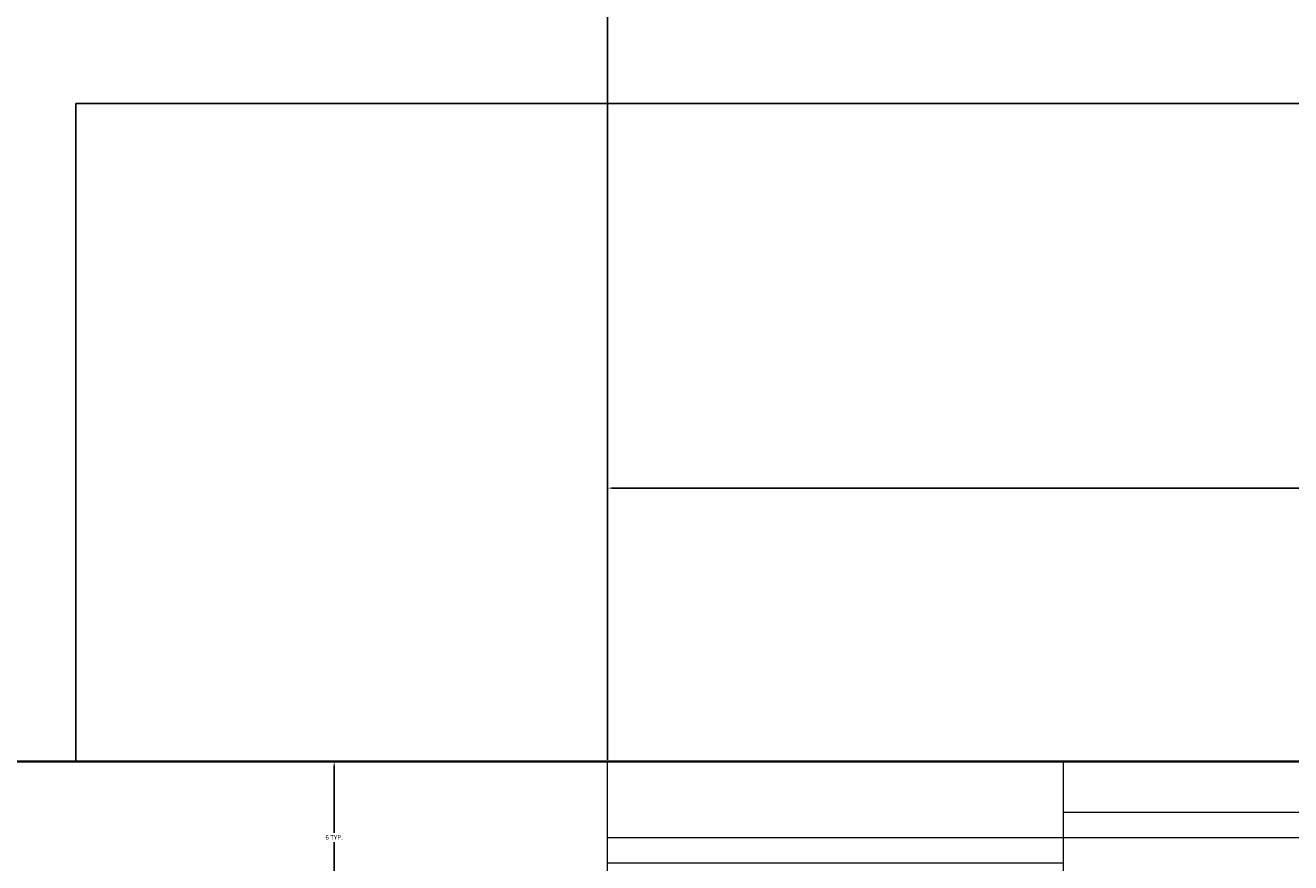
# Model space of a CAD drawing. Units: feet. Extents: x 105 to 1094, y -88 to 588.
# Tile 55 of 59: x 649 to 699, y 437 to 470. Entities that reach past the tile are written whole.
import ezdxf

# ---------------------------------------------------------------- set-up
doc = ezdxf.new("R2010")
doc.units = ezdxf.units.FT
doc.header["$MEASUREMENT"] = 0
for name, color, linetype, lineweight in [('A-ANNO-DIMS', 2, 'Continuous', 18), ('A-FLOR-PROJ', 8, 'Continuous', 25), ('A-GLAZ', 4, 'Continuous', 18), ('A-WALL', 7, 'Continuous', 35)]:
    doc.layers.add(name, color=color, linetype=linetype, lineweight=lineweight)
doc.styles.get("Standard").update_dxf_attribs({"font": 'arial.ttf'})
doc.dimstyles.get("Standard").update_dxf_attribs({"dimtxt": 0.18, "dimasz": 0.18, "dimexe": 0.18, "dimexo": 0.0625, "dimgap": 0.09, "dimtad": 0, "dimtih": 1, "dimtoh": 1, "dimdec": 4, "dimzin": 0, "dimdsep": 46, "dimtxsty": 'Standard', "dimcen": 0.09, "dimadec": 0, "dimazin": 0, "dimtfac": 1, "dimtdec": 4, "dimtofl": 0, "dimtmove": 0, "dimatfit": 3, "dimfxl": 1, "dimtolj": 1, "dimtzin": 0, "dimarcsym": 0})

# ---------------------------------------------------------------- blocks, each defined once
blk = doc.blocks.new('WIN-FOUR-LIGHT-WIDE')
for p, q in [((0, 0), (0, 6)), ((18, 0), (18, 6)), ((18, 4), (36, 4)), ((0, 3), (72, 3)), ((0, 2), (18, 2))]:
    blk.add_line(p, q)
blk = doc.blocks.new('*D12')
at = {"layer": 'A-ANNO-DIMS', "color": 0, "lineweight": -2, "transparency": 16777216}
for p, q in [((671.688, 441.144), (671.688, 452.061)), ((671.868, 451.881), (705.69, 451.881)), ((743.508, 451.881), (709.687, 451.881)), ((743.688, 441.144), (743.688, 452.061))]:
    blk.add_line(p, q, dxfattribs=at)
at = {"layer": 'A-ANNO-DIMS', "color": 0, "transparency": 16777216}
for points in [[(671.868, 451.911), (671.868, 451.851), (671.688, 451.881)], [(743.508, 451.911), (743.508, 451.851), (743.688, 451.881)]]:
    blk.add_solid(points, dxfattribs=at)
at = {"layer": 'Defpoints', "color": 0, "transparency": 16777216}
for p in [(743.688, 451.881), (671.688, 441.081), (743.688, 441.081)]:
    blk.add_point(p, dxfattribs=at)
at = {"layer": 'A-ANNO-DIMS', "color": 0, "transparency": 16777216, "insert": (707.688, 451.881), "char_height": 0.18, "attachment_point": 5}
blk.add_mtext('\\A1;WIDE 4-LIGHT WINDOW 72 TYP.', dxfattribs=at)
blk = doc.blocks.new('*D13')
at = {"layer": 'A-ANNO-DIMS', "color": 0, "lineweight": -2, "transparency": 16777216}
for p, q in [((671.626, 441.081), (660.708, 441.081)), ((660.888, 440.901), (660.888, 438.263)), ((660.888, 435.261), (660.888, 437.899)), ((671.626, 435.081), (660.708, 435.081))]:
    blk.add_line(p, q, dxfattribs=at)
at = {"layer": 'A-ANNO-DIMS', "color": 0, "transparency": 16777216}
for points in [[(660.858, 440.901), (660.918, 440.901), (660.888, 441.081)], [(660.858, 435.261), (660.918, 435.261), (660.888, 435.081)]]:
    blk.add_solid(points, dxfattribs=at)
at = {"layer": 'Defpoints', "color": 0, "transparency": 16777216}
for p in [(660.888, 441.081), (671.688, 441.081), (671.688, 435.081)]:
    blk.add_point(p, dxfattribs=at)
at = {"layer": 'A-ANNO-DIMS', "color": 0, "transparency": 16777216, "insert": (660.888, 438.081), "char_height": 0.18, "attachment_point": 5}
blk.add_mtext('\\A1;6 TYP.', dxfattribs=at)
blk = doc.blocks.new('*D21')
at = {"layer": 'A-ANNO-DIMS', "color": 0, "lineweight": -2, "transparency": 16777216}
for p, q in [((849.626, 543.081), (105.458, 543.081)), ((105.638, 542.901), (105.638, 250.263)), ((105.638, -42.739), (105.638, 249.899)), ((849.626, -42.919), (105.458, -42.919))]:
    blk.add_line(p, q, dxfattribs=at)
at = {"layer": 'A-ANNO-DIMS', "color": 0, "transparency": 16777216}
for points in [[(105.608, 542.901), (105.668, 542.901), (105.638, 543.081)], [(105.608, -42.739), (105.668, -42.739), (105.638, -42.919)]]:
    blk.add_solid(points, dxfattribs=at)
at = {"layer": 'Defpoints', "color": 0, "transparency": 16777216}
for p in [(105.638, 543.081), (849.688, 543.081), (849.688, -42.919)]:
    blk.add_point(p, dxfattribs=at)
at = {"layer": 'A-ANNO-DIMS', "color": 0, "transparency": 16777216, "insert": (105.638, 250.081), "char_height": 0.18, "attachment_point": 5}
blk.add_mtext('\\A1;586', dxfattribs=at)
blk = doc.blocks.new('*D41')
at = {"layer": 'A-ANNO-DIMS', "color": 0, "lineweight": -2, "transparency": 16777216}
for p, q in [((646.688, 441.144), (646.688, 588.311)), ((671.688, 441.144), (671.688, 588.311)), ((646.868, 588.131), (658.967, 588.131)), ((671.508, 588.131), (659.409, 588.131))]:
    blk.add_line(p, q, dxfattribs=at)
at = {"layer": 'A-ANNO-DIMS', "color": 0, "transparency": 16777216}
for points in [[(646.868, 588.161), (646.868, 588.101), (646.688, 588.131)], [(671.508, 588.161), (671.508, 588.101), (671.688, 588.131)]]:
    blk.add_solid(points, dxfattribs=at)
at = {"layer": 'Defpoints', "color": 0, "transparency": 16777216}
for p in [(671.688, 588.131), (646.688, 441.081), (671.688, 441.081)]:
    blk.add_point(p, dxfattribs=at)
at = {"layer": 'A-ANNO-DIMS', "color": 0, "transparency": 16777216, "insert": (659.188, 588.131), "char_height": 0.18, "attachment_point": 5}
blk.add_mtext('\\A1;25', dxfattribs=at)

msp = doc.modelspace()

# ---------------------------------------------------------------- linework, layer by layer
at = {"layer": 'A-FLOR-PROJ'}
for p, q in [((650.6883, 467.0812), (650.6883, 441.0812)), ((760.6883, 467.0812), (650.6883, 467.0812))]:
    msp.add_line(p, q, dxfattribs=at)
at = {"layer": 'A-WALL'}
msp.add_line((760.6883, 441.0812), (646.6883, 441.0812), dxfattribs=at)

# ---------------------------------------------------------------- block references
at = {"layer": 'A-GLAZ'}
msp.add_blockref('WIN-FOUR-LIGHT-WIDE', (671.688, 435.081), dxfattribs=at)

# ---------------------------------------------------------------- dimensions: what is measured, and where the dimension line sits
at = {"layer": 'A-ANNO-DIMS'}
dim = msp.add_linear_dim(base=(671.6883, 588.1312), p1=(646.6883, 441.0812), p2=(671.6883, 441.0812), dimstyle='Standard', override={"dimdec": 0, "dimlfac": 1, "dimrnd": 0, "dimzin": 0, "dimdsep": 46, "dimlunit": 2}, dxfattribs=at)
dim.commit()
dim.dimension.update_dxf_attribs({"geometry": '*D41', "text_midpoint": (659.1883, 588.1312)})
dim = msp.add_linear_dim(base=(105.6383, 543.0812), p1=(849.6883, -42.9188), p2=(849.6883, 543.0812), angle=90, dimstyle='Standard', override={"dimdec": 0, "dimlfac": 1, "dimrnd": 0, "dimzin": 0, "dimdsep": 46, "dimlunit": 2}, dxfattribs=at)
dim.commit()
dim.dimension.update_dxf_attribs({"geometry": '*D21', "text_midpoint": (105.6383, 250.0812)})
dim = msp.add_linear_dim(base=(743.6883, 451.8812), p1=(671.6883, 441.0812), p2=(743.6883, 441.0812), text='WIDE 4-LIGHT WINDOW <> TYP.', dimstyle='Standard', override={"dimdec": 0, "dimlfac": 1, "dimrnd": 0, "dimzin": 0, "dimdsep": 46, "dimlunit": 2}, dxfattribs=at)
dim.commit()
dim.dimension.update_dxf_attribs({"geometry": '*D12', "text_midpoint": (707.6883, 451.8812)})
dim = msp.add_linear_dim(base=(660.8883, 441.0812), p1=(671.6883, 435.0812), p2=(671.6883, 441.0812), angle=90, text='<> TYP.', dimstyle='Standard', override={"dimdec": 0, "dimlfac": 1, "dimrnd": 0, "dimzin": 0, "dimdsep": 46, "dimlunit": 2}, dxfattribs=at)
dim.commit()
dim.dimension.update_dxf_attribs({"geometry": '*D13', "text_midpoint": (660.8883, 438.0812)})

doc.saveas('drawing.dxf')
